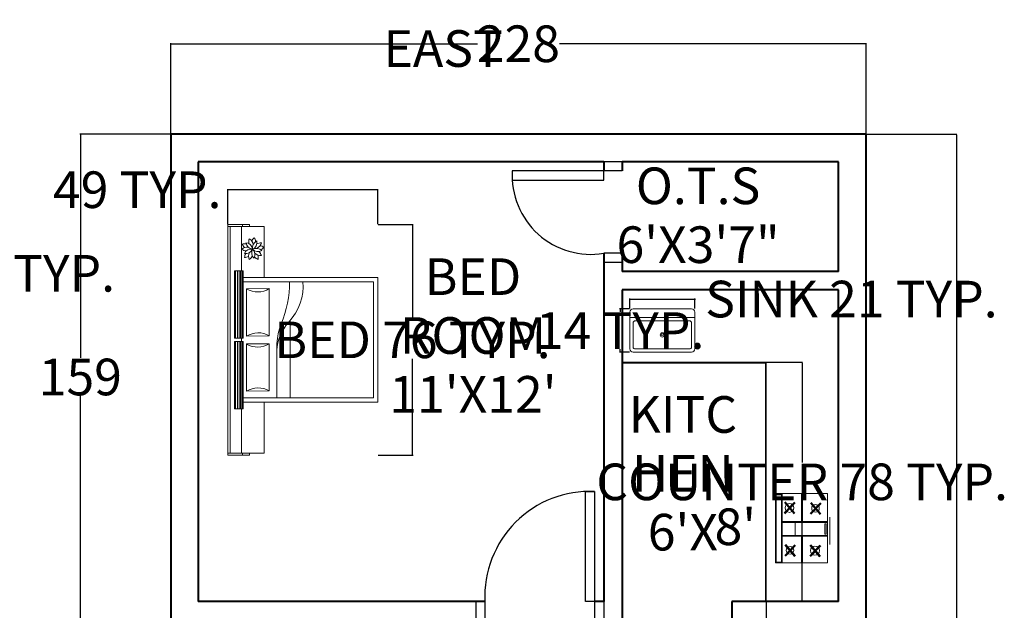
# Model space of a CAD drawing. Units: inches. Extents: x -124 to 612, y -69 to 524.
# Tile 9 of 9: x 287 to 610, y 329 to 523. Entities that reach past the tile are written whole.
import ezdxf
from ezdxf.enums import TextEntityAlignment as Align

# ---------------------------------------------------------------- set-up
doc = ezdxf.new("R2010")
doc.units = ezdxf.units.IN
doc.header["$MEASUREMENT"] = 0
for name, color, linetype, lineweight in [('A-ANNO-DIMS', 2, 'Continuous', 18), ('A-ANNO-TEXT', 1, 'Continuous', 18), ('A-AREA-IDEN', 1, 'Continuous', 18), ('A-DOOR', 4, 'Continuous', 25), ('A-EQPM', 9, 'Continuous', 18), ('A-FLOR-CASE', 8, 'Continuous', 18), ('A-FLOR-FIXT', 9, 'Continuous', 18), ('A-FURN', 8, 'Continuous', 18), ('A-WALL', 7, 'Continuous', 40)]:
    doc.layers.add(name, color=color, linetype=linetype, lineweight=lineweight)
doc.styles.add('ATTR', font='romans.shx', dxfattribs={"width": 0.8, "height": 1.075})
doc.styles.get("Standard").update_dxf_attribs({"font": 'arial.ttf'})
doc.dimstyles.get("Standard").update_dxf_attribs({"dimtxt": 12, "dimasz": 0.18, "dimexe": 0.18, "dimexo": 0.0625, "dimgap": 0.09, "dimtad": 0, "dimtih": 1, "dimtoh": 1, "dimdec": 0, "dimzin": 0, "dimdsep": 46, "dimlunit": 4, "dimtxsty": 'Standard', "dimcen": 0.09, "dimadec": 0, "dimazin": 0, "dimtfac": 1, "dimtdec": 0, "dimtofl": 0, "dimtmove": 0, "dimatfit": 3, "dimfxl": 1, "dimtolj": 1, "dimtzin": 0, "dimarcsym": 0})

# ---------------------------------------------------------------- blocks, each defined once
blk = doc.blocks.new('A$C7BDD1693')
for p, q in [((0, 2.068), (0, 1.768)), ((0, 2.068), (1.615, 2.068)), ((0.03, 1.768), (0.03, 2.068)), ((0.03, 2.038), (0.64, 2.038)), ((0.64, 2.038), (1.565, 2.038)), ((1.565, 2.038), (1.615, 2.038)), ((1.615, 2.068), (2.54, 2.068)), ((1.615, 2.038), (2.54, 2.038)), ((2.54, 2.068), (3.18, 2.068)), ((3.15, 2.038), (2.54, 2.038)), ((3.15, 1.768), (3.15, 2.068)), ((3.18, 2.068), (3.18, 1.768)), ((0.64, 1.978), (1.565, 1.978)), ((0.64, 1.978), (0.64, 1.858)), ((0.64, 1.963), (1.565, 1.963)), ((0.64, 1.937), (1.565, 1.937)), ((0.64, 1.912), (1.565, 1.912)), ((1.565, 1.978), (1.565, 1.858)), ((1.615, 1.978), (1.615, 1.858)), ((1.615, 1.978), (2.54, 1.978)), ((1.615, 1.963), (2.54, 1.963)), ((1.615, 1.937), (2.54, 1.937)), ((1.615, 1.912), (2.54, 1.912)), ((2.54, 1.978), (2.54, 1.858)), ((0.03, 1.868), (0, 1.868)), ((0, 1.768), (0.03, 1.768)), ((0.03, 1.88), (0.64, 1.88)), ((0.03, 1.768), (0.03, 1.568)), ((0.03, 1.768), (0.03, 1.568)), ((0.64, 1.893), (1.565, 1.893)), ((0.64, 1.877), (1.565, 1.877)), ((0.64, 1.866), (1.565, 1.866)), ((0.64, 1.858), (1.565, 1.858)), ((0.73, 1.568), (0.73, 1.858)), ((0.79, 1.858), (0.79, 0.06)), ((1.533, 1.81), (0.883, 1.81)), ((0.883, 1.81), (0.887, 1.498)), ((1.537, 1.498), (1.533, 1.81)), ((1.565, 1.88), (1.615, 1.88)), ((1.615, 1.893), (2.54, 1.893)), ((1.615, 1.877), (2.54, 1.877)), ((1.615, 1.866), (2.54, 1.866)), ((1.615, 1.858), (2.54, 1.858)), ((2.291, 1.81), (1.641, 1.81)), ((1.641, 1.81), (1.646, 1.498)), ((2.296, 1.498), (2.291, 1.81)), ((2.39, 1.858), (2.39, 0.06)), ((2.45, 1.568), (2.45, 1.858)), ((3.15, 1.88), (2.54, 1.88)), ((3.15, 1.868), (3.18, 1.868)), ((3.15, 1.568), (3.15, 1.768)), ((3.18, 1.768), (3.15, 1.768)), ((0.03, 1.568), (0.73, 1.568)), ((0.73, 1.568), (0.73, 0)), ((0.887, 1.498), (1.537, 1.498)), ((1.646, 1.498), (2.296, 1.498)), ((3.15, 1.568), (2.45, 1.568)), ((2.45, 1.568), (2.45, 0)), ((1.54, 1.392), (0.79, 1.392)), ((1.848, 1.209), (0.79, 1.209)), ((0.73, 0), (2.45, 0)), ((0.79, 0.06), (2.39, 0.06))]:
    blk.add_line(p, q)
for centre, radius, start, end in [((0.626, 1.65), 0.303, 329.8722, 31.8713), ((1.794, 1.658), 0.303, 149.8722, 211.8713), ((1.384, 1.65), 0.303, 329.8722, 31.8713), ((2.553, 1.658), 0.303, 149.8722, 211.8713), ((2.74, 1.667), 0.115, 63.1324, 112.6013), ((2.798, 1.845), 0.125, 215.1301, 245.4931), ((2.879, 1.849), 0.155, 184.2105, 205.3514), ((2.726, 1.74), 0.0968, 57.5086, 91.2476), ((2.884, 1.823), 0.106, 170.7761, 244.5159), ((2.743, 1.749), 0.098, 347.0447, 68.2473), ((2.938, 1.802), 0.125, 143.1301, 173.4932), ((2.751, 1.802), 0.115, 351.1324, 40.6013), ((2.944, 1.713), 0.106, 98.7761, 172.5159), ((2.83, 1.825), 0.098, 275.0447, 356.2473), ((2.967, 1.726), 0.155, 112.2105, 133.3514), ((2.883, 1.833), 0.115, 279.1324, 328.6013), ((2.817, 1.838), 0.0968, 345.5086, 19.2476), ((2.941, 1.655), 0.125, 71.1301, 101.4931), ((2.791, 1.624), 0.0968, 129.5086, 163.2476), ((2.735, 1.803), 0.155, 256.2105, 277.3514), ((2.788, 1.643), 0.098, 59.0447, 140.2473), ((2.761, 1.8), 0.106, 242.7761, 316.5159), ((2.865, 1.615), 0.115, 135.1324, 184.6013), ((2.713, 1.725), 0.125, 287.1301, 317.4932), ((2.903, 1.653), 0.098, 131.0447, 212.2473), ((2.745, 1.676), 0.106, 314.7761, 28.5159), ((2.858, 1.622), 0.106, 26.7761, 100.5159), ((2.929, 1.765), 0.098, 203.0447, 284.2473), ((2.953, 1.718), 0.115, 207.1324, 256.6013), ((2.802, 1.607), 0.125, 359.1301, 29.4932), ((2.937, 1.782), 0.0968, 273.5086, 307.2476), ((2.877, 1.605), 0.155, 40.2105, 61.3514), ((2.921, 1.65), 0.0968, 201.5086, 235.2476), ((2.734, 1.652), 0.155, 328.2105, 349.3514)]:
    blk.add_arc(centre, radius, start, end)
for centre, major_axis, ratio, start_param, end_param in [((1.413, 0.552), (0, -0.842), 0.84, 2.512571, 3.097265), ((1.474, 0.023), (0, -1.371), 0.84, 2.845884, 3.083884), ((2.394, 3.329), (0, -2.112), 0.84, -0.336035, -0.002349), ((2.261, 1.856), (0.259, -0.793), 0.868451, -0.988378, -0.183496)]:
    blk.add_ellipse(centre, major_axis=major_axis, ratio=ratio, start_param=start_param, end_param=end_param)
blk = doc.blocks.new('A$C0FBA78B1')
for p, q in [((750, 589), (0, 589)), ((0, 589), (0, 24)), ((0, 518), (0, 584)), ((0, 584), (745, 584)), ((7, 524), (7, 580)), ((7, 580), (738, 580)), ((738, 580), (738, 524)), ((745, 584), (745, 518)), ((750, 589), (750, 24)), ((745, 518), (0, 518)), ((738, 524), (7, 524)), ((70, 381), (192, 486)), ((189, 370), (73, 481)), ((74, 376), (195, 482)), ((193, 374), (77, 485)), ((78, 372), (199, 478)), ((197, 378), (80, 489)), ((289, 518), (289, 305)), ((296, 518), (296, 24)), ((439, 518), (439, 297)), ((447, 518), (447, 305)), ((531, 387), (653, 492)), ((650, 376), (533, 487)), ((535, 383), (656, 488)), ((653, 380), (537, 491)), ((538, 379), (660, 484)), ((657, 384), (541, 495)), ((296, 376), (438, 376)), ((0, 305), (289, 305)), ((0, 297), (289, 297)), ((67, 110), (189, 216)), ((190, 103), (74, 214)), ((194, 107), (77, 218)), ((289, 297), (289, 24)), ((439, 297), (439, 24)), ((447, 305), (750, 305)), ((447, 297), (447, 24)), ((447, 297), (750, 297)), ((186, 99), (70, 210)), ((71, 106), (192, 212)), ((75, 102), (196, 207)), ((525, 104), (646, 210)), ((644, 93), (527, 204)), ((529, 100), (650, 205)), ((647, 97), (531, 208)), ((532, 96), (654, 201)), ((651, 101), (535, 212)), ((0, 24), (750, 24)), ((494, 0), (198, 0)), ((311, 41), (311, 54)), ((311, 54), (424, 54)), ((424, 41), (311, 41)), ((424, 54), (424, 41))]:
    blk.add_line(p, q)
for centre, radius in [((136, 431), 41.2), ((596, 437), 48.4), ((133, 161), 48.4), ((590, 155), 41.2)]:
    blk.add_circle(centre, radius)
blk = doc.blocks.new("30'' Sink Single PV")
blk.add_line((-15, -3.999996), (15, -3.999996))
for points in [[(-13.5, 0), (13.5, 0)], [(-15, -18.499996), (-15, -1.5)], [(15, -1.5), (15, -18.499996)], [(-13.5, -17.499996), (-13.5, -6.499996)], [(-12.5, -5.499996), (12.5, -5.499996)], [(13.5, -6.499996), (13.5, -17.499996)], [(13.5, -19.999996), (-13.5, -19.999996)], [(12.5, -18.499996), (-12.5, -18.499996)]]:
    blk.add_lwpolyline(points)
for radius in [1, 0.5]:
    blk.add_circle((0, -11.999996), radius)
for centre, radius, start, end in [((-13.5, -1.5), 1.5, 90, 180), ((13.5, -1.5), 1.5, 0, 90), ((-12.5, -6.499996), 1, 90, 180), ((12.5, -6.499996), 1, 0, 90), ((-12.5, -17.499996), 1, 180, 270), ((12.5, -17.499996), 1, 270, 0), ((-13.5, -18.499996), 1.5, 180, 270), ((13.5, -18.499996), 1.5, 270, 0)]:
    blk.add_arc(centre, radius, start, end)
at = {"style": 'ATTR', "width": 0.8, "flags": 9}
blk.add_attdef('ESTCODE', (0, 0), '', height=0.006, dxfattribs=at)
blk = doc.blocks.new('DOOR-36IN-SINGLE')
for p, q in [((0, 6), (0, 0)), ((3, 6), (3, 0)), ((39, 6), (39, 0)), ((42, 6), (42, 0))]:
    blk.add_line(p, q)
blk.add_lwpolyline([(39, 6), (36, 6), (36, 42), (39, 42)], close=True)
blk.add_arc((37.5, 7.5), 34.53, 87.5104, 182.4896)
blk = doc.blocks.new('DOOR-30IN-OTS')
for p, q in [((36.04, 33), (30.04, 33)), ((36.04, 30), (30.04, 30)), ((36.04, 3), (30.04, 3)), ((36.04, 0), (30.04, 0))]:
    blk.add_line(p, q)
blk.add_lwpolyline([(30.04, 30), (0.04, 30), (0.04, 27), (30.04, 27)], close=True)
blk.add_arc((25.84, 28.5), 25.84, 176.6726, 279.353)
blk = doc.blocks.new('COUNTER-L-KITCHEN')
for p, q in [((47.3, 78.3), (0, 78.3)), ((47, 78), (0, 78)), ((47, 0), (47, 78)), ((47.3, 0), (47.3, 78.3))]:
    blk.add_line(p, q)
blk = doc.blocks.new('*D21')
at = {"layer": 'A-ANNO-DIMS', "color": 0, "lineweight": -2, "transparency": 16777216}
for p, q in [((405, 455.59), (416.47, 455.59)), ((416.29, 455.41), (416.29, 423.98)), ((416.29, 380.12), (416.29, 411.55)), ((405, 379.94), (416.47, 379.94))]:
    blk.add_line(p, q, dxfattribs=at)
at = {"layer": 'A-ANNO-DIMS', "color": 0, "transparency": 16777216}
for points in [[(416.26, 455.41), (416.32, 455.41), (416.29, 455.59)], [(416.26, 380.12), (416.32, 380.12), (416.29, 379.94)]]:
    blk.add_solid(points, dxfattribs=at)
at = {"layer": 'Defpoints', "color": 0, "transparency": 16777216}
for p in [(404.94, 455.59), (416.29, 455.59), (404.94, 379.94)]:
    blk.add_point(p, dxfattribs=at)
at = {"layer": 'A-ANNO-DIMS', "color": 0, "transparency": 16777216, "insert": (416.29, 417.77), "char_height": 12, "attachment_point": 5}
blk.add_mtext('\\A1;BED 76 TYP.', dxfattribs=at)
blk = doc.blocks.new('*D22')
at = {"layer": 'A-ANNO-DIMS', "color": 0, "lineweight": -2, "transparency": 16777216}
for p, q in [((355.75, 466.94), (355.57, 466.94)), ((355.75, 455.65), (355.75, 467.12)), ((404.76, 466.94), (355.93, 466.94)), ((404.94, 455.65), (404.94, 467.12))]:
    blk.add_line(p, q, dxfattribs=at)
at = {"layer": 'A-ANNO-DIMS', "color": 0, "transparency": 16777216}
for points in [[(355.93, 466.97), (355.93, 466.91), (355.75, 466.94)], [(404.76, 466.97), (404.76, 466.91), (404.94, 466.94)]]:
    blk.add_solid(points, dxfattribs=at)
at = {"layer": 'Defpoints', "color": 0, "transparency": 16777216}
for p in [(355.75, 466.94), (355.75, 455.59), (404.94, 455.59)]:
    blk.add_point(p, dxfattribs=at)
at = {"layer": 'A-ANNO-DIMS', "color": 0, "transparency": 16777216, "insert": (326.03, 466.94), "char_height": 12, "attachment_point": 5}
blk.add_mtext('\\A1;49 TYP.', dxfattribs=at)
blk = doc.blocks.new('*D33')
at = {"layer": 'A-ANNO-DIMS', "color": 0, "lineweight": -2, "transparency": 16777216}
for p, q in [((487.57, 427.98), (487.57, 431.3)), ((487.75, 431.12), (508.71, 431.12)), ((508.89, 427.98), (508.89, 431.3)), ((508.89, 431.12), (509.07, 431.12))]:
    blk.add_line(p, q, dxfattribs=at)
at = {"layer": 'A-ANNO-DIMS', "color": 0, "transparency": 16777216}
for points in [[(487.75, 431.15), (487.75, 431.09), (487.57, 431.12)], [(508.71, 431.15), (508.71, 431.09), (508.89, 431.12)]]:
    blk.add_solid(points, dxfattribs=at)
at = {"layer": 'Defpoints', "color": 0, "transparency": 16777216}
for p in [(508.89, 431.12), (487.57, 427.92), (508.89, 427.92)]:
    blk.add_point(p, dxfattribs=at)
at = {"layer": 'A-ANNO-DIMS', "color": 0, "transparency": 16777216, "insert": (560.23, 431.12), "char_height": 12, "attachment_point": 5}
blk.add_mtext('\\A1;SINK 21 TYP.', dxfattribs=at)
blk = doc.blocks.new('*D34')
at = {"layer": 'A-ANNO-DIMS', "color": 0, "lineweight": -2, "transparency": 16777216}
for p, q in [((487.51, 427.92), (484.2, 427.92)), ((484.38, 427.74), (484.38, 426.93)), ((487.51, 413.7), (484.2, 413.7)), ((484.38, 413.88), (484.38, 414.69))]:
    blk.add_line(p, q, dxfattribs=at)
at = {"layer": 'A-ANNO-DIMS', "color": 0, "transparency": 16777216}
for points in [[(484.35, 427.74), (484.41, 427.74), (484.38, 427.92)], [(484.35, 413.88), (484.41, 413.88), (484.38, 413.7)]]:
    blk.add_solid(points, dxfattribs=at)
at = {"layer": 'Defpoints', "color": 0, "transparency": 16777216}
for p in [(484.38, 427.92), (487.57, 427.92), (487.57, 413.7)]:
    blk.add_point(p, dxfattribs=at)
at = {"layer": 'A-ANNO-DIMS', "color": 0, "transparency": 16777216, "insert": (484.38, 420.81), "char_height": 12, "attachment_point": 5}
blk.add_mtext('\\A1;14 TYP.', dxfattribs=at)
blk = doc.blocks.new('*D37')
at = {"layer": 'A-ANNO-DIMS', "color": 0, "lineweight": -2, "transparency": 16777216}
for p, q in [((121.9, 444.97), (121.9, 439.38)), ((158.35, 444.97), (158.35, 439.38)), ((122.08, 439.56), (158.17, 439.56)), ((158.35, 439.56), (158.53, 439.56))]:
    blk.add_line(p, q, dxfattribs=at)
at = {"layer": 'A-ANNO-DIMS', "color": 0, "transparency": 16777216}
for points in [[(122.08, 439.59), (122.08, 439.53), (121.9, 439.56)], [(158.17, 439.59), (158.17, 439.53), (158.35, 439.56)]]:
    blk.add_solid(points, dxfattribs=at)
at = {"layer": 'Defpoints', "color": 0, "transparency": 16777216}
for p in [(121.9, 445.03), (158.35, 445.03), (158.35, 439.56)]:
    blk.add_point(p, dxfattribs=at)
at = {"layer": 'A-ANNO-DIMS', "color": 0, "transparency": 16777216, "insert": (241.79, 439.56), "char_height": 12, "attachment_point": 5}
blk.add_mtext('\\A1;O.T.S. DOOR 36 TYP.', dxfattribs=at)
blk = doc.blocks.new('*D43')
at = {"layer": 'A-ANNO-DIMS', "color": 0, "lineweight": -2, "transparency": 16777216}
for p, q in [((532.38, 410.4), (544.24, 410.4)), ((544.06, 410.22), (544.06, 377.55)), ((544.06, 332.28), (544.06, 364.96)), ((532.38, 332.1), (544.24, 332.1))]:
    blk.add_line(p, q, dxfattribs=at)
at = {"layer": 'A-ANNO-DIMS', "color": 0, "transparency": 16777216}
for points in [[(544.03, 410.22), (544.09, 410.22), (544.06, 410.4)], [(544.03, 332.28), (544.09, 332.28), (544.06, 332.1)]]:
    blk.add_solid(points, dxfattribs=at)
at = {"layer": 'Defpoints', "color": 0, "transparency": 16777216}
for p in [(532.32, 410.4), (544.06, 410.4), (532.32, 332.1)]:
    blk.add_point(p, dxfattribs=at)
at = {"layer": 'A-ANNO-DIMS', "color": 0, "transparency": 16777216, "insert": (544.06, 371.25), "char_height": 12, "attachment_point": 5}
blk.add_mtext('\\A1;COUNTER 78 TYP.', dxfattribs=at)
blk = doc.blocks.new('*D44')
at = {"layer": 'A-ANNO-DIMS', "color": 0, "lineweight": -2, "transparency": 16777216}
for p, q in [((485.02, 332.04), (485.02, 320.18)), ((532.32, 332.04), (532.32, 320.18)), ((485.2, 320.36), (532.14, 320.36)), ((532.32, 320.36), (532.5, 320.36))]:
    blk.add_line(p, q, dxfattribs=at)
at = {"layer": 'A-ANNO-DIMS', "color": 0, "transparency": 16777216}
for points in [[(485.2, 320.39), (485.2, 320.33), (485.02, 320.36)], [(532.14, 320.39), (532.14, 320.33), (532.32, 320.36)]]:
    blk.add_solid(points, dxfattribs=at)
at = {"layer": 'Defpoints', "color": 0, "transparency": 16777216}
for p in [(485.02, 332.1), (532.32, 332.1), (532.32, 320.36)]:
    blk.add_point(p, dxfattribs=at)
at = {"layer": 'A-ANNO-DIMS', "color": 0, "transparency": 16777216, "insert": (562.03, 320.36), "char_height": 12, "attachment_point": 5}
blk.add_mtext('\\A1;47 TYP.', dxfattribs=at)
blk = doc.blocks.new('*D49')
at = {"layer": 'A-ANNO-DIMS', "color": 0, "lineweight": -2, "transparency": 16777216}
for p, q in [((337.02, 485.17), (337.02, 514.93)), ((337.2, 514.75), (437.56, 514.75)), ((564.84, 514.75), (464.48, 514.75)), ((565.02, 485.17), (565.02, 514.93))]:
    blk.add_line(p, q, dxfattribs=at)
at = {"layer": 'A-ANNO-DIMS', "color": 0, "transparency": 16777216}
for points in [[(337.2, 514.78), (337.2, 514.72), (337.02, 514.75)], [(564.84, 514.78), (564.84, 514.72), (565.02, 514.75)]]:
    blk.add_solid(points, dxfattribs=at)
at = {"layer": 'Defpoints', "color": 0, "transparency": 16777216}
for p in [(565.02, 514.75), (337.02, 485.1), (565.02, 485.1)]:
    blk.add_point(p, dxfattribs=at)
at = {"layer": 'A-ANNO-DIMS', "color": 0, "transparency": 16777216, "insert": (451.02, 514.75), "char_height": 12, "attachment_point": 5}
blk.add_mtext('\\A1;228', dxfattribs=at)
blk = doc.blocks.new('*D50')
at = {"layer": 'A-ANNO-DIMS', "color": 0, "lineweight": -2, "transparency": 16777216}
for p, q in [((565.08, 485.1), (594.85, 485.1)), ((594.67, 484.92), (594.67, 233.32)), ((594.67, -30.72), (594.67, 220.89)), ((564.78, -30.9), (594.85, -30.9))]:
    blk.add_line(p, q, dxfattribs=at)
at = {"layer": 'A-ANNO-DIMS', "color": 0, "transparency": 16777216}
for points in [[(594.64, 484.92), (594.7, 484.92), (594.67, 485.1)], [(594.64, -30.72), (594.7, -30.72), (594.67, -30.9)]]:
    blk.add_solid(points, dxfattribs=at)
at = {"layer": 'Defpoints', "color": 0, "transparency": 16777216}
for p in [(565.02, 485.1), (594.67, 485.1), (564.72, -30.9)]:
    blk.add_point(p, dxfattribs=at)
at = {"layer": 'A-ANNO-DIMS', "color": 0, "transparency": 16777216, "insert": (594.67, 227.1), "char_height": 12, "attachment_point": 5}
blk.add_mtext('\\A1;516', dxfattribs=at)
blk = doc.blocks.new('*D60')
at = {"layer": 'A-ANNO-DIMS', "color": 0, "lineweight": -2, "transparency": 16777216}
for p, q in [((336.95, 485.1), (307.19, 485.1)), ((307.37, 484.92), (307.37, 411.82)), ((307.37, 326.28), (307.37, 399.39)), ((345.95, 326.1), (307.19, 326.1))]:
    blk.add_line(p, q, dxfattribs=at)
at = {"layer": 'A-ANNO-DIMS', "color": 0, "transparency": 16777216}
for points in [[(307.34, 484.92), (307.4, 484.92), (307.37, 485.1)], [(307.34, 326.28), (307.4, 326.28), (307.37, 326.1)]]:
    blk.add_solid(points, dxfattribs=at)
at = {"layer": 'Defpoints', "color": 0, "transparency": 16777216}
for p in [(307.37, 485.1), (337.02, 485.1), (346.02, 326.1)]:
    blk.add_point(p, dxfattribs=at)
at = {"layer": 'A-ANNO-DIMS', "color": 0, "transparency": 16777216, "insert": (307.37, 405.6), "char_height": 12, "attachment_point": 5}
blk.add_mtext('\\A1;159', dxfattribs=at)

msp = doc.modelspace()

# ---------------------------------------------------------------- linework, layer by layer
at = {"layer": 'A-WALL'}
for p, q in [((565.0169, 485.1047), (337.0169, 485.1047)), ((337.0169, 485.1047), (337.0169, -31.1953)), ((565.0169, -31.1953), (565.0169, 485.1047)), ((479.0169, 476.1047), (346.0169, 476.1047)), ((346.0169, 476.1047), (346.0169, 332.1047)), ((479.0169, 476.1047), (479.0169, 473.1047)), ((556.0169, 476.1047), (485.0169, 476.1047)), ((485.0169, 476.1047), (485.0169, 473.1047)), ((556.0169, 440.1047), (556.0169, 476.1047)), ((479.0169, 446.1047), (479.0169, 332.1047)), ((485.0169, 446.1047), (485.0169, 440.1047)), ((556.0169, 440.1047), (485.0169, 440.1047)), ((556.0169, 434.1047), (485.0169, 434.1047)), ((485.0169, 434.1047), (485.0169, 332.1047)), ((556.0169, 332.1047), (556.0169, 434.1047)), ((440.0169, 332.1047), (346.0169, 332.1047)), ((479.0169, 332.1047), (476.0169, 332.1047)), ((485.0169, 332.1047), (485.0169, 326.1047)), ((556.0169, 332.1047), (521.0169, 332.1047)), ((521.0169, 332.1047), (521.0169, 326.1047))]:
    msp.add_line(p, q, dxfattribs=at)

# ---------------------------------------------------------------- block references
at = {"layer": 'A-DOOR'}
for name, p in [('DOOR-30IN-OTS', (448.9736, 443.1046)), ('DOOR-36IN-SINGLE', (437.0166, 326.1046))]:
    msp.add_blockref(name, p, dxfattribs=at)
at = {"layer": 'A-EQPM', "xscale": 0.030262411053157, "yscale": 0.030262411053157, "zscale": 0.030262411053157, "rotation": 90}
msp.add_blockref('A$C0FBA78B1', (553.1413, 344.691), dxfattribs=at)
at = {"layer": 'A-FLOR-CASE'}
msp.add_blockref('COUNTER-L-KITCHEN', (485.0166, 332.1046), dxfattribs=at)
at = {"layer": 'A-FLOR-FIXT', "xscale": 0.710634528886296, "yscale": 0.710634528886296, "zscale": 0.710634528886296}
msp.add_blockref("30'' Sink Single PV", (498.233, 427.915, 10.4529), dxfattribs=at)
at = {"layer": 'A-FURN', "xscale": 23.78825355168716, "yscale": 23.78825355168716, "zscale": 23.78825355168716, "rotation": 90}
msp.add_blockref('A$C7BDD1693', (404.9425, 379.9429), dxfattribs=at)

# ---------------------------------------------------------------- texts
at = {"layer": 'A-ANNO-TEXT'}
msp.add_text('EAST', height=12, dxfattribs=at).set_placement((426.3695, 507.1865), align=Align.CENTER)
at = {"layer": 'A-AREA-IDEN'}
for s, p in [('O.T.S', (509.9465, 462.2148)), ('6\'X3\'7"', (509.9465, 442.9379)), ('BED', (436.1229, 432.4638)), ('ROOM', (436.1229, 413.1869)), ("11'X12'", (436.1229, 393.9099)), ('KITC', (504.9588, 387.3212)), ('HEN', (504.9588, 368.0443)), ("8'", (522.1685, 350.5445)), ("6'X", (504.9588, 348.7673))]:
    msp.add_text(s, height=12, dxfattribs=at).set_placement(p, align=Align.CENTER)

# ---------------------------------------------------------------- dimensions: what is measured, and where the dimension line sits
at = {"layer": 'A-ANNO-DIMS'}
dim = msp.add_linear_dim(base=(565.0169, 514.7547), p1=(337.0169, 485.1047), p2=(565.0169, 485.1047), dimstyle='Standard', override={"dimdec": 0, "dimlfac": 1, "dimrnd": 0, "dimzin": 0, "dimdsep": 46, "dimlunit": 2}, dxfattribs=at)
dim.commit()
dim.dimension.update_dxf_attribs({"geometry": '*D49', "text_midpoint": (451.0169, 514.7547)})
for base, p1, p2, picture, middle in [((307.3669, 485.1047), (346.0169, 326.1047), (337.0169, 485.1047), '*D60', (307.3669, 405.6047)), ((594.6669, 485.1047), (564.7169, -30.8953), (565.0169, 485.1047), '*D50', (594.6669, 227.1047))]:
    dim = msp.add_linear_dim(base=base, p1=p1, p2=p2, angle=90, dimstyle='Standard', override={"dimdec": 0, "dimlfac": 1, "dimrnd": 0, "dimzin": 0, "dimdsep": 46, "dimlunit": 2}, dxfattribs=at)
    dim.commit()
    dim.dimension.update_dxf_attribs({"geometry": picture, "text_midpoint": middle})
for base, p1, p2, angle, text, picture, middle in [((355.7511, 466.9366), (404.9425, 455.5896), (355.7511, 455.5896), 180, '<> TYP.', '*D22', (326.0336, 466.9366)), ((416.2895, 455.5896), (404.9425, 379.9429), (404.9425, 455.5896), 90, 'BED <> TYP.', '*D21', (416.2895, 417.7663)), ((484.3756, 427.9193), (487.5735, 413.7023), (487.5735, 427.9193), 90, '<> TYP.', '*D34', (484.3756, 420.8108)), ((544.0619, 410.4047), (532.3169, 332.1047), (532.3169, 410.4047), 90, 'COUNTER <> TYP.', '*D43', (544.0619, 371.2547))]:
    dim = msp.add_linear_dim(base=base, p1=p1, p2=p2, angle=angle, text=text, dimstyle='Standard', override={"dimdec": 0, "dimlfac": 1, "dimrnd": 0, "dimzin": 0, "dimdsep": 46, "dimlunit": 2}, dxfattribs=at)
    dim.commit()
    dim.dimension.update_dxf_attribs({"geometry": picture, "text_midpoint": middle})
for base, p1, p2, text, picture, middle in [((158.3513, 439.5607), (121.8956, 445.0291), (158.3513, 445.0291), 'O.T.S. DOOR <> TYP.', '*D37', (241.7905, 439.5607)), ((508.8925, 431.1171), (487.5735, 427.9193), (508.8925, 427.9193), 'SINK <> TYP.', '*D33', (560.2321, 431.1171)), ((532.3169, 320.3597), (485.0169, 332.1047), (532.3169, 332.1047), '<> TYP.', '*D44', (562.0344, 320.3597))]:
    dim = msp.add_linear_dim(base=base, p1=p1, p2=p2, text=text, dimstyle='Standard', override={"dimdec": 0, "dimlfac": 1, "dimrnd": 0, "dimzin": 0, "dimdsep": 46, "dimlunit": 2}, dxfattribs=at)
    dim.commit()
    dim.dimension.update_dxf_attribs({"geometry": picture, "text_midpoint": middle})

doc.saveas('drawing.dxf')
